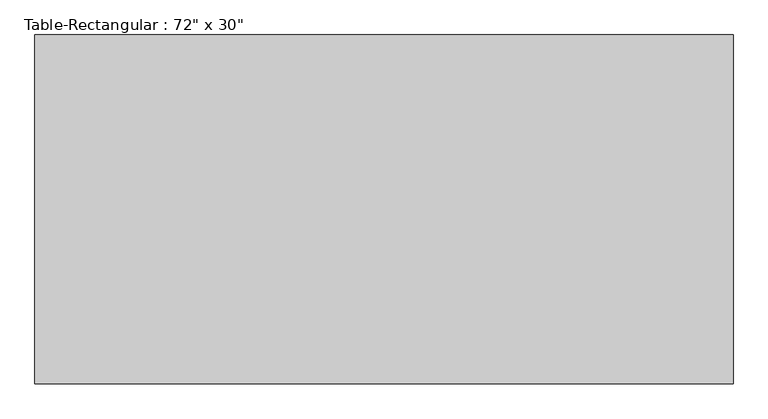
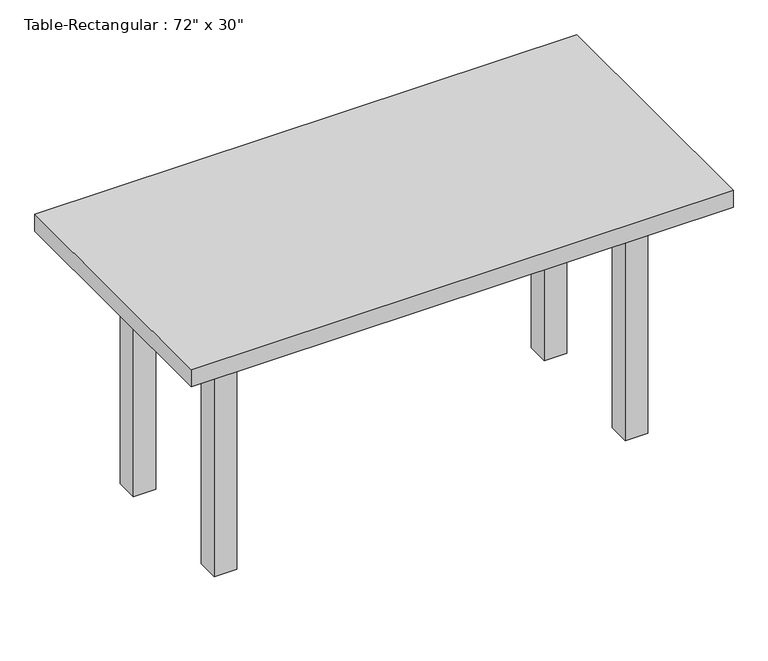
"""IFC4 building model written with IfcOpenShell, lengths in millimetres: furniture geometry."""

from ifc_helpers import new_model, si_unit, frame, origin, origin_with_axes, place, context, project, spatial, polyline, outline, extrude, source, transform, mapped, element, save


def furniture_d900495b(model_context):
    return source(origin(), model_context, "Body", "SweptSolid", [
        extrude(outline(polyline([(546.1, 190.5), (546.1, 165.1), (-546.1, 165.1), (-546.1, 190.5), (546.1, 190.5)])), frame((0.0, 0.0, 609.6), z_axis=(0.0, 0.0, 1.0), x_axis=(1.0, 0.0, 0.0)), (0.0, 0.0, 1.0), 101.6),
        extrude(outline(polyline([(546.1, -190.5), (-546.1, -190.5), (-546.1, -165.1), (546.1, -165.1), (546.1, -190.5)])), frame((0.0, 0.0, 609.6), z_axis=(0.0, 0.0, 1.0), x_axis=(1.0, 0.0, 0.0)), (0.0, 0.0, 1.0), 101.6),
        extrude(outline(polyline([(-558.8, -165.1), (-584.2, -165.1), (-584.2, 165.1), (-558.8, 165.1), (-558.8, -165.1)])), frame((0.0, 0.0, 609.6), z_axis=(0.0, 0.0, 1.0), x_axis=(1.0, 0.0, 0.0)), (0.0, 0.0, 1.0), 101.6),
        extrude(outline(polyline([(558.8, -165.1), (558.8, 165.1), (584.2, 165.1), (584.2, -165.1), (558.8, -165.1)])), frame((0.0, 0.0, 609.6), z_axis=(0.0, 0.0, 1.0), x_axis=(1.0, 0.0, 0.0)), (0.0, 0.0, 1.0), 101.6),
        extrude(outline(polyline([(762.0, 381.0), (762.0, -381.0), (-762.0, -381.0), (-762.0, 381.0), (762.0, 381.0)])), frame((0.0, 0.0, 711.2), z_axis=(0.0, 0.0, 1.0), x_axis=(1.0, 0.0, 0.0)), (0.0, 0.0, 1.0), 50.8),
        extrude(outline(polyline([(-546.1, 228.6), (-546.1, 165.1), (-609.6, 165.1), (-609.6, 228.6), (-546.1, 228.6)])), origin_with_axes(), (0.0, 0.0, 1.0), 711.2),
        extrude(outline(polyline([(546.1, 228.6), (609.6, 228.6), (609.6, 165.1), (546.1, 165.1), (546.1, 228.6)])), origin_with_axes(), (0.0, 0.0, 1.0), 711.2),
        extrude(outline(polyline([(-546.1, -228.6), (-609.6, -228.6), (-609.6, -165.1), (-546.1, -165.1), (-546.1, -228.6)])), origin_with_axes(), (0.0, 0.0, 1.0), 711.2),
        extrude(outline(polyline([(546.1, -228.6), (546.1, -165.1), (609.6, -165.1), (609.6, -228.6), (546.1, -228.6)])), origin_with_axes(), (0.0, 0.0, 1.0), 711.2),
    ])


if __name__ == "__main__":
    model = new_model("IFC4")
    model_context = context("Model", 3, world=origin())
    ifc_project = project(units=[si_unit("LENGTHUNIT", "METRE", prefix="MILLI")], contexts=[model_context])
    site = spatial("IfcSite", under=ifc_project)
    building = spatial("IfcBuilding", under=site)
    placement = place(None, origin())
    furniture_shape = furniture_d900495b(model_context)
    element("IfcFurniture", 1, ObjectType="Table-Rectangular : 72\" x 30\"", at=placement, inside=building, context=model_context, shape_type="MappedRepresentation", body=[
        mapped(furniture_shape, transform((0.0, 0.0, 0.0), x_axis=(1.0, 0.0, 0.0), y_axis=(0.0, 1.0, 0.0), z_axis=(0.0, 0.0, 1.0))),
    ])
    save(model, "model.ifc")

# Revit data of these elements
# Type "Table-Rectangular : 72\" x 30\""
#   Assembly Code = "E2020200"
#   Height = 2' - 6"
#   Length = 5' - 0"
#   Width = 2' - 6"
#   Base Material = Birch
#   Top Material = Birch
#   Default Elevation = 0
# Element 1 (IfcFurniture, "Table-Rectangular : 72\" x 30\"")
#   Materials on its faces: "Birch"
# Materials
#   "Birch": class "Wood", colour RGB 224 178 126, transparency 0, Description = "Betula Alleghaniensis", Cost = 0
